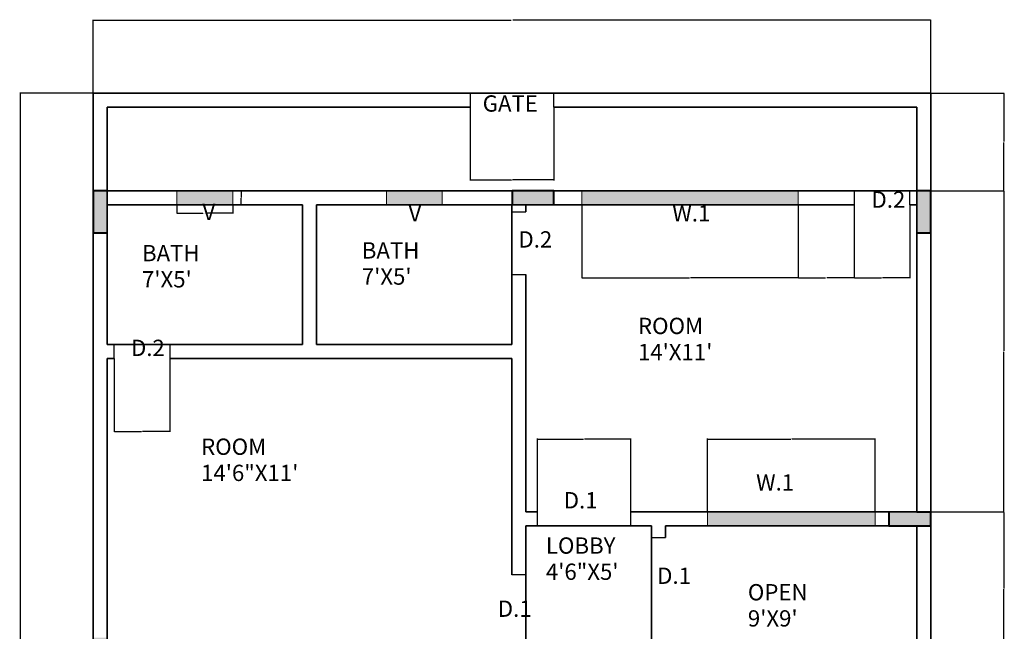
# Model space of a CAD drawing. Units: inches. Extents: x 2156 to 3149, y 1513 to 2286.
# Tile 2 of 5: x 2156 to 2579, y 1937 to 2200. Entities that reach past the tile are written whole.
import ezdxf

# ---------------------------------------------------------------- set-up
doc = ezdxf.new("R2010")
doc.units = ezdxf.units.IN
for name, color, linetype, lineweight in [('A-ANNO-DIMS', 2, 'Continuous', 18), ('A-ANNO-TEXT', 7, 'Continuous', 18), ('A-AREA-IDEN', 7, 'Continuous', 18), ('A-COLS', 7, 'Continuous', 40), ('A-COLS-PATT', 18, 'Continuous', 13), ('A-DOOR', 3, 'Continuous', 25), ('A-GLAZ', 4, 'Continuous', 18), ('A-GLAZ-PATT', 252, 'Continuous', 13), ('A-SITE-GATE', 3, 'Continuous', 25), ('A-SITE-WALL', 7, 'Continuous', 35), ('A-WALL', 7, 'Continuous', 35)]:
    doc.layers.add(name, color=color, linetype=linetype, lineweight=lineweight)
doc.styles.get("Standard").update_dxf_attribs({"font": 'arial.ttf'})
doc.dimstyles.get("Standard").update_dxf_attribs({"dimtxt": 0.18, "dimasz": 0.18, "dimexe": 0.18, "dimexo": 0.0625, "dimgap": 0.09, "dimtad": 0, "dimtih": 1, "dimtoh": 1, "dimdec": 4, "dimzin": 0, "dimdsep": 46, "dimtxsty": 'Standard', "dimcen": 0.09, "dimadec": 0, "dimazin": 0, "dimtfac": 1, "dimtdec": 4, "dimtofl": 0, "dimtmove": 0, "dimatfit": 3, "dimfxl": 1, "dimtolj": 1, "dimtzin": 0, "dimarcsym": 0})

# ---------------------------------------------------------------- blocks, each defined once
blk = doc.blocks.new('COL-6X18-PLAN')
for p, q in [((6, 18), (0, 18)), ((0, 18), (0, 0)), ((0, 0), (6, 0))]:
    blk.add_line(p, q)
blk = doc.blocks.new('VENT-24-PLAN')
for p, q in [((0, 0), (0, 6)), ((0, 6), (24, 6)), ((24, 6), (24, 0))]:
    blk.add_line(p, q)
blk = doc.blocks.new('*D9')
at = {"layer": 'A-ANNO-DIMS', "color": 0, "lineweight": -2, "transparency": 16777216}
for p, q in [((2223.92, 2120.47), (2223.92, 2116.76)), ((2247.92, 2120.47), (2247.92, 2116.76)), ((2224.1, 2116.94), (2235.02, 2116.94)), ((2247.74, 2116.94), (2236.82, 2116.94))]:
    blk.add_line(p, q, dxfattribs=at)
at = {"layer": 'A-ANNO-DIMS', "color": 0, "transparency": 16777216}
for points in [[(2224.1, 2116.97), (2224.1, 2116.91), (2223.92, 2116.94)], [(2247.74, 2116.97), (2247.74, 2116.91), (2247.92, 2116.94)]]:
    blk.add_solid(points, dxfattribs=at)
at = {"layer": 'Defpoints', "color": 0, "transparency": 16777216}
for p in [(2223.92, 2120.54), (2247.92, 2120.54), (2247.92, 2116.94)]:
    blk.add_point(p, dxfattribs=at)
at = {"layer": 'A-ANNO-DIMS', "color": 0, "transparency": 16777216, "insert": (2235.92, 2116.94), "char_height": 0.18, "attachment_point": 5}
blk.add_mtext('\\A1;VENT 24 TYP.', dxfattribs=at)
blk = doc.blocks.new('*D10')
at = {"layer": 'A-ANNO-DIMS', "color": 0, "lineweight": -2, "transparency": 16777216}
for p, q in [((2247.98, 2126.54), (2251.7, 2126.54)), ((2251.52, 2126.36), (2251.52, 2123.72)), ((2247.98, 2120.54), (2251.7, 2120.54)), ((2251.52, 2120.72), (2251.52, 2123.35))]:
    blk.add_line(p, q, dxfattribs=at)
at = {"layer": 'A-ANNO-DIMS', "color": 0, "transparency": 16777216}
for points in [[(2251.49, 2126.36), (2251.55, 2126.36), (2251.52, 2126.54)], [(2251.49, 2120.72), (2251.55, 2120.72), (2251.52, 2120.54)]]:
    blk.add_solid(points, dxfattribs=at)
at = {"layer": 'Defpoints', "color": 0, "transparency": 16777216}
for p in [(2247.92, 2126.54), (2251.52, 2126.54), (2247.92, 2120.54)]:
    blk.add_point(p, dxfattribs=at)
at = {"layer": 'A-ANNO-DIMS', "color": 0, "transparency": 16777216, "insert": (2251.52, 2123.54), "char_height": 0.18, "attachment_point": 5}
blk.add_mtext('\\A1;6 TYP.', dxfattribs=at)
blk = doc.blocks.new('*D19')
at = {"layer": 'A-ANNO-DIMS', "color": 0, "lineweight": -2, "transparency": 16777216}
for p, q in [((2187.92, 2168.6), (2187.92, 2200.07)), ((2188.1, 2199.89), (2367.63, 2199.89)), ((2547.74, 2199.89), (2368.21, 2199.89)), ((2547.92, 2168.6), (2547.92, 2200.07))]:
    blk.add_line(p, q, dxfattribs=at)
at = {"layer": 'A-ANNO-DIMS', "color": 0, "transparency": 16777216}
for points in [[(2188.1, 2199.92), (2188.1, 2199.86), (2187.92, 2199.89)], [(2547.74, 2199.92), (2547.74, 2199.86), (2547.92, 2199.89)]]:
    blk.add_solid(points, dxfattribs=at)
at = {"layer": 'Defpoints', "color": 0, "transparency": 16777216}
for p in [(2547.92, 2199.89), (2187.92, 2168.54), (2547.92, 2168.54)]:
    blk.add_point(p, dxfattribs=at)
at = {"layer": 'A-ANNO-DIMS', "color": 0, "transparency": 16777216, "insert": (2367.92, 2199.89), "char_height": 0.18, "attachment_point": 5}
blk.add_mtext('\\A1;360', dxfattribs=at)
blk = doc.blocks.new('*D24')
at = {"layer": 'A-ANNO-DIMS', "color": 0, "lineweight": -2, "transparency": 16777216}
for p, q in [((2187.86, 2168.54), (2156.39, 2168.54)), ((2156.57, 2168.36), (2156.57, 1856.72)), ((2156.57, 1544.72), (2156.57, 1856.35)), ((2187.86, 1544.54), (2156.39, 1544.54))]:
    blk.add_line(p, q, dxfattribs=at)
at = {"layer": 'A-ANNO-DIMS', "color": 0, "transparency": 16777216}
for points in [[(2156.54, 2168.36), (2156.6, 2168.36), (2156.57, 2168.54)], [(2156.54, 1544.72), (2156.6, 1544.72), (2156.57, 1544.54)]]:
    blk.add_solid(points, dxfattribs=at)
at = {"layer": 'Defpoints', "color": 0, "transparency": 16777216}
for p in [(2156.57, 2168.54), (2187.92, 2168.54), (2187.92, 1544.54)]:
    blk.add_point(p, dxfattribs=at)
at = {"layer": 'A-ANNO-DIMS', "color": 0, "transparency": 16777216, "insert": (2156.57, 1856.54), "char_height": 0.18, "attachment_point": 5}
blk.add_mtext('\\A1;624', dxfattribs=at)
blk = doc.blocks.new('*D29')
at = {"layer": 'A-ANNO-DIMS', "color": 0, "lineweight": -2, "transparency": 16777216}
for p, q in [((2547.98, 1988.54), (2579.45, 1988.54)), ((2579.27, 1988.36), (2579.27, 1955.72)), ((2579.27, 1922.72), (2579.27, 1955.35)), ((2433.98, 1922.54), (2579.45, 1922.54))]:
    blk.add_line(p, q, dxfattribs=at)
at = {"layer": 'A-ANNO-DIMS', "color": 0, "transparency": 16777216}
for points in [[(2579.24, 1988.36), (2579.3, 1988.36), (2579.27, 1988.54)], [(2579.24, 1922.72), (2579.3, 1922.72), (2579.27, 1922.54)]]:
    blk.add_solid(points, dxfattribs=at)
at = {"layer": 'Defpoints', "color": 0, "transparency": 16777216}
for p in [(2547.92, 1988.54), (2579.27, 1988.54), (2433.92, 1922.54)]:
    blk.add_point(p, dxfattribs=at)
at = {"layer": 'A-ANNO-DIMS', "color": 0, "transparency": 16777216, "insert": (2579.27, 1955.54), "char_height": 0.18, "attachment_point": 5}
blk.add_mtext('\\A1;66', dxfattribs=at)
blk = doc.blocks.new('*D30')
at = {"layer": 'A-ANNO-DIMS', "color": 0, "lineweight": -2, "transparency": 16777216}
for p, q in [((2547.98, 2126.54), (2579.45, 2126.54)), ((2579.27, 2126.36), (2579.27, 2057.72)), ((2579.27, 1988.72), (2579.27, 2057.35)), ((2547.98, 1988.54), (2579.45, 1988.54))]:
    blk.add_line(p, q, dxfattribs=at)
at = {"layer": 'A-ANNO-DIMS', "color": 0, "transparency": 16777216}
for points in [[(2579.24, 2126.36), (2579.3, 2126.36), (2579.27, 2126.54)], [(2579.24, 1988.72), (2579.3, 1988.72), (2579.27, 1988.54)]]:
    blk.add_solid(points, dxfattribs=at)
at = {"layer": 'Defpoints', "color": 0, "transparency": 16777216}
for p in [(2547.92, 2126.54), (2579.27, 2126.54), (2547.92, 1988.54)]:
    blk.add_point(p, dxfattribs=at)
at = {"layer": 'A-ANNO-DIMS', "color": 0, "transparency": 16777216, "insert": (2579.27, 2057.54), "char_height": 0.18, "attachment_point": 5}
blk.add_mtext('\\A1;138', dxfattribs=at)
blk = doc.blocks.new('*D31')
at = {"layer": 'A-ANNO-DIMS', "color": 0, "lineweight": -2, "transparency": 16777216}
for p, q in [((2547.98, 2168.54), (2579.45, 2168.54)), ((2579.27, 2168.36), (2579.27, 2147.72)), ((2579.27, 2126.72), (2579.27, 2147.36)), ((2547.98, 2126.54), (2579.45, 2126.54))]:
    blk.add_line(p, q, dxfattribs=at)
at = {"layer": 'A-ANNO-DIMS', "color": 0, "transparency": 16777216}
for points in [[(2579.24, 2168.36), (2579.3, 2168.36), (2579.27, 2168.54)], [(2579.24, 2126.72), (2579.3, 2126.72), (2579.27, 2126.54)]]:
    blk.add_solid(points, dxfattribs=at)
at = {"layer": 'Defpoints', "color": 0, "transparency": 16777216}
for p in [(2547.92, 2168.54), (2579.27, 2168.54), (2547.92, 2126.54)]:
    blk.add_point(p, dxfattribs=at)
at = {"layer": 'A-ANNO-DIMS', "color": 0, "transparency": 16777216, "insert": (2579.27, 2147.54), "char_height": 0.18, "attachment_point": 5}
blk.add_mtext('\\A1;42', dxfattribs=at)
blk = doc.blocks.new('*D32')
at = {"layer": 'A-ANNO-DIMS', "color": 0, "lineweight": -2, "transparency": 16777216}
for p, q in [((2349.92, 2162.47), (2349.92, 2131.01)), ((2385.92, 2162.47), (2385.92, 2131.01)), ((2350.1, 2131.19), (2367.7, 2131.19)), ((2385.74, 2131.19), (2368.14, 2131.19))]:
    blk.add_line(p, q, dxfattribs=at)
at = {"layer": 'A-ANNO-DIMS', "color": 0, "transparency": 16777216}
for points in [[(2350.1, 2131.22), (2350.1, 2131.16), (2349.92, 2131.19)], [(2385.74, 2131.22), (2385.74, 2131.16), (2385.92, 2131.19)]]:
    blk.add_solid(points, dxfattribs=at)
at = {"layer": 'Defpoints', "color": 0, "transparency": 16777216}
for p in [(2349.92, 2162.54), (2385.92, 2162.54), (2349.92, 2131.19)]:
    blk.add_point(p, dxfattribs=at)
at = {"layer": 'A-ANNO-DIMS', "color": 0, "transparency": 16777216, "insert": (2367.92, 2131.19), "char_height": 0.18, "attachment_point": 5}
blk.add_mtext('\\A1;36', dxfattribs=at)
blk = doc.blocks.new('*D33')
at = {"layer": 'A-ANNO-DIMS', "color": 0, "lineweight": -2, "transparency": 16777216}
for p, q in [((2397.92, 2120.47), (2397.92, 2089.01)), ((2490.92, 2120.47), (2490.92, 2089.01)), ((2398.1, 2089.19), (2444.2, 2089.19)), ((2490.74, 2089.19), (2444.64, 2089.19))]:
    blk.add_line(p, q, dxfattribs=at)
at = {"layer": 'A-ANNO-DIMS', "color": 0, "transparency": 16777216}
for points in [[(2398.1, 2089.22), (2398.1, 2089.16), (2397.92, 2089.19)], [(2490.74, 2089.22), (2490.74, 2089.16), (2490.92, 2089.19)]]:
    blk.add_solid(points, dxfattribs=at)
at = {"layer": 'Defpoints', "color": 0, "transparency": 16777216}
for p in [(2397.92, 2120.54), (2490.92, 2120.54), (2397.92, 2089.19)]:
    blk.add_point(p, dxfattribs=at)
at = {"layer": 'A-ANNO-DIMS', "color": 0, "transparency": 16777216, "insert": (2444.42, 2089.19), "char_height": 0.18, "attachment_point": 5}
blk.add_mtext('\\A1;93', dxfattribs=at)
blk = doc.blocks.new('*D34')
at = {"layer": 'A-ANNO-DIMS', "color": 0, "lineweight": -2, "transparency": 16777216}
for p, q in [((2490.92, 2120.47), (2490.92, 2089.01)), ((2514.92, 2120.47), (2514.92, 2089.01)), ((2491.1, 2089.19), (2502.7, 2089.19)), ((2514.74, 2089.19), (2503.14, 2089.19))]:
    blk.add_line(p, q, dxfattribs=at)
at = {"layer": 'A-ANNO-DIMS', "color": 0, "transparency": 16777216}
for points in [[(2491.1, 2089.22), (2491.1, 2089.16), (2490.92, 2089.19)], [(2514.74, 2089.22), (2514.74, 2089.16), (2514.92, 2089.19)]]:
    blk.add_solid(points, dxfattribs=at)
at = {"layer": 'Defpoints', "color": 0, "transparency": 16777216}
for p in [(2490.92, 2120.54), (2514.92, 2120.54), (2490.92, 2089.19)]:
    blk.add_point(p, dxfattribs=at)
at = {"layer": 'A-ANNO-DIMS', "color": 0, "transparency": 16777216, "insert": (2502.92, 2089.19), "char_height": 0.18, "attachment_point": 5}
blk.add_mtext('\\A1;24', dxfattribs=at)
blk = doc.blocks.new('*D35')
at = {"layer": 'A-ANNO-DIMS', "color": 0, "lineweight": -2, "transparency": 16777216}
for p, q in [((2514.92, 2120.47), (2514.92, 2089.01)), ((2538.92, 2120.47), (2538.92, 2089.01)), ((2515.1, 2089.19), (2526.7, 2089.19)), ((2538.74, 2089.19), (2527.14, 2089.19))]:
    blk.add_line(p, q, dxfattribs=at)
at = {"layer": 'A-ANNO-DIMS', "color": 0, "transparency": 16777216}
for points in [[(2515.1, 2089.22), (2515.1, 2089.16), (2514.92, 2089.19)], [(2538.74, 2089.22), (2538.74, 2089.16), (2538.92, 2089.19)]]:
    blk.add_solid(points, dxfattribs=at)
at = {"layer": 'Defpoints', "color": 0, "transparency": 16777216}
for p in [(2514.92, 2120.54), (2538.92, 2120.54), (2514.92, 2089.19)]:
    blk.add_point(p, dxfattribs=at)
at = {"layer": 'A-ANNO-DIMS', "color": 0, "transparency": 16777216, "insert": (2526.92, 2089.19), "char_height": 0.18, "attachment_point": 5}
blk.add_mtext('\\A1;24', dxfattribs=at)
blk = doc.blocks.new('*D36')
at = {"layer": 'A-ANNO-DIMS', "color": 0, "lineweight": -2, "transparency": 16777216}
for p, q in [((2451.92, 1988.6), (2451.92, 2020.07)), ((2452.1, 2019.89), (2487.7, 2019.89)), ((2523.74, 2019.89), (2488.14, 2019.89)), ((2523.92, 1988.6), (2523.92, 2020.07))]:
    blk.add_line(p, q, dxfattribs=at)
at = {"layer": 'A-ANNO-DIMS', "color": 0, "transparency": 16777216}
for points in [[(2452.1, 2019.92), (2452.1, 2019.86), (2451.92, 2019.89)], [(2523.74, 2019.92), (2523.74, 2019.86), (2523.92, 2019.89)]]:
    blk.add_solid(points, dxfattribs=at)
at = {"layer": 'Defpoints', "color": 0, "transparency": 16777216}
for p in [(2523.92, 2019.89), (2451.92, 1988.54), (2523.92, 1988.54)]:
    blk.add_point(p, dxfattribs=at)
at = {"layer": 'A-ANNO-DIMS', "color": 0, "transparency": 16777216, "insert": (2487.92, 2019.89), "char_height": 0.18, "attachment_point": 5}
blk.add_mtext('\\A1;72', dxfattribs=at)
blk = doc.blocks.new('*D37')
at = {"layer": 'A-ANNO-DIMS', "color": 0, "lineweight": -2, "transparency": 16777216}
for p, q in [((2378.92, 1988.6), (2378.92, 2020.07)), ((2379.1, 2019.89), (2398.7, 2019.89)), ((2418.74, 2019.89), (2399.14, 2019.89)), ((2418.92, 1988.6), (2418.92, 2020.07))]:
    blk.add_line(p, q, dxfattribs=at)
at = {"layer": 'A-ANNO-DIMS', "color": 0, "transparency": 16777216}
for points in [[(2379.1, 2019.92), (2379.1, 2019.86), (2378.92, 2019.89)], [(2418.74, 2019.92), (2418.74, 2019.86), (2418.92, 2019.89)]]:
    blk.add_solid(points, dxfattribs=at)
at = {"layer": 'Defpoints', "color": 0, "transparency": 16777216}
for p in [(2418.92, 2019.89), (2378.92, 1988.54), (2418.92, 1988.54)]:
    blk.add_point(p, dxfattribs=at)
at = {"layer": 'A-ANNO-DIMS', "color": 0, "transparency": 16777216, "insert": (2398.92, 2019.89), "char_height": 0.18, "attachment_point": 5}
blk.add_mtext('\\A1;40', dxfattribs=at)
blk = doc.blocks.new('*D38')
at = {"layer": 'A-ANNO-DIMS', "color": 0, "lineweight": -2, "transparency": 16777216}
for p, q in [((2196.92, 2054.47), (2196.92, 2023.01)), ((2220.92, 2054.47), (2220.92, 2023.01)), ((2197.1, 2023.19), (2208.7, 2023.19)), ((2220.74, 2023.19), (2209.14, 2023.19))]:
    blk.add_line(p, q, dxfattribs=at)
at = {"layer": 'A-ANNO-DIMS', "color": 0, "transparency": 16777216}
for points in [[(2197.1, 2023.22), (2197.1, 2023.16), (2196.92, 2023.19)], [(2220.74, 2023.22), (2220.74, 2023.16), (2220.92, 2023.19)]]:
    blk.add_solid(points, dxfattribs=at)
at = {"layer": 'Defpoints', "color": 0, "transparency": 16777216}
for p in [(2196.92, 2054.54), (2220.92, 2054.54), (2196.92, 2023.19)]:
    blk.add_point(p, dxfattribs=at)
at = {"layer": 'A-ANNO-DIMS', "color": 0, "transparency": 16777216, "insert": (2208.92, 2023.19), "char_height": 0.18, "attachment_point": 5}
blk.add_mtext('\\A1;24', dxfattribs=at)

msp = doc.modelspace()

# ---------------------------------------------------------------- hatches: boundary and pattern name
at = {"layer": 'A-COLS-PATT'}
h = msp.add_hatch(color=256, dxfattribs=at)
h.dxf.hatch_style = 1
h.paths.add_polyline_path([(2193.921, 2120.536), (2193.921, 2126.536), (2187.921, 2126.536), (2187.921, 2108.536), (2193.921, 2108.536)])
h.paths.add_polyline_path([(2385.921, 2126.536), (2367.921, 2126.536), (2367.921, 2120.536), (2373.921, 2120.536), (2385.921, 2120.536)])
h.paths.add_polyline_path([(2547.921, 2126.536), (2541.921, 2126.536), (2541.921, 2108.536), (2547.921, 2108.536)])
h.paths.add_polyline_path([(2547.921, 1988.536), (2541.921, 1988.536), (2541.921, 1982.536), (2547.921, 1982.536)])
h.paths.add_polyline_path([(2541.921, 1988.536), (2529.921, 1988.536), (2529.921, 1982.536), (2541.921, 1982.536)])
h.paths.add_polyline_path([(2373.921, 1922.536), (2367.921, 1922.536), (2355.921, 1922.536), (2355.921, 1916.536), (2373.921, 1916.536)])
h.paths.add_polyline_path([(2193.921, 1934.536), (2187.921, 1934.536), (2187.921, 1916.536), (2193.921, 1916.536)])
h.paths.add_polyline_path([(2433.921, 1880.536), (2427.921, 1880.536), (2427.921, 1871.536), (2427.921, 1862.536), (2433.921, 1862.536)])
h.paths.add_polyline_path([(2241.921, 1772.536), (2235.921, 1772.536), (2235.921, 1760.536), (2235.921, 1754.536), (2241.921, 1754.536)])
h.paths.add_polyline_path([(2443.921, 1760.536), (2433.921, 1760.536), (2427.921, 1760.536), (2425.921, 1760.536), (2425.921, 1754.536), (2443.921, 1754.536)])
h.paths.add_polyline_path([(2547.921, 1760.536), (2541.921, 1760.536), (2541.921, 1754.536), (2541.921, 1742.536), (2547.921, 1742.536)])
at = {"layer": 'A-GLAZ-PATT'}
h = msp.add_hatch(color=256, dxfattribs=at)
h.dxf.hatch_style = 1
h.paths.add_polyline_path([(2490.921, 2126.536), (2397.921, 2126.536), (2397.921, 2120.536), (2490.921, 2120.536)])
h.paths.add_polyline_path([(2337.921, 2126.536), (2313.921, 2126.536), (2313.921, 2120.536), (2325.921, 2120.536), (2337.921, 2120.536)])
h.paths.add_polyline_path([(2247.921, 2126.536), (2223.921, 2126.536), (2223.921, 2120.536), (2235.921, 2120.536), (2247.921, 2120.536)])
h.paths.add_polyline_path([(2241.921, 1891.536), (2235.921, 1891.536), (2235.921, 1831.536), (2241.921, 1831.536), (2241.921, 1861.536)])
h.paths.add_polyline_path([(2235.921, 1922.536), (2193.921, 1922.536), (2193.921, 1916.536), (2235.921, 1916.536)])
h.paths.add_polyline_path([(2505.921, 1874.536), (2469.921, 1874.536), (2469.921, 1868.536), (2505.921, 1868.536)])
h.paths.add_polyline_path([(2523.921, 1988.536), (2451.921, 1988.536), (2451.921, 1982.536), (2523.921, 1982.536)])
h.paths.add_polyline_path([(2307.921, 1760.536), (2289.921, 1760.536), (2289.921, 1754.536), (2298.921, 1754.536), (2307.921, 1754.536)])
h.paths.add_polyline_path([(2422.921, 1760.536), (2404.921, 1760.536), (2404.921, 1754.536), (2413.921, 1754.536), (2422.921, 1754.536)])

# ---------------------------------------------------------------- linework, layer by layer
at = {"layer": 'A-COLS'}
msp.add_line((2541.921, 1988.536), (2547.921, 1988.536), dxfattribs=at)
at = {"layer": 'A-DOOR'}
for p, q in [((2538.921, 2126.536), (2514.921, 2126.536)), ((2514.921, 2126.536), (2514.921, 2120.536)), ((2538.921, 2120.536), (2538.921, 2126.536)), ((2367.921, 2117.536), (2373.921, 2117.536)), ((2367.921, 2117.536), (2367.921, 2090.536)), ((2367.921, 2090.536), (2373.921, 2090.536)), ((2196.921, 2054.536), (2196.921, 2060.536)), ((2196.921, 2060.536), (2214.921, 2060.536)), ((2214.921, 2060.536), (2220.921, 2060.536)), ((2220.921, 2060.536), (2220.921, 2054.536)), ((2378.921, 1982.536), (2378.921, 1988.536)), ((2418.921, 1982.536), (2418.921, 1988.536)), ((2427.921, 1977.536), (2433.921, 1977.536)), ((2373.921, 1961.536), (2367.921, 1961.536)), ((2373.921, 1925.536), (2373.921, 1961.536))]:
    msp.add_line(p, q, dxfattribs=at)
at = {"layer": 'A-GLAZ'}
for p, q in [((2397.921, 2120.536), (2397.921, 2126.536)), ((2490.921, 2120.536), (2490.921, 2126.536)), ((2451.921, 1982.536), (2451.921, 1988.536)), ((2523.921, 1982.536), (2523.921, 1988.536))]:
    msp.add_line(p, q, dxfattribs=at)
at = {"layer": 'A-SITE-GATE'}
for p, q in [((2385.921, 2168.536), (2349.921, 2168.536)), ((2349.921, 2168.536), (2349.921, 2162.536)), ((2385.921, 2162.536), (2385.921, 2168.536))]:
    msp.add_line(p, q, dxfattribs=at)
at = {"layer": 'A-SITE-WALL'}
for p, q in [((2187.921, 2168.536), (2547.921, 2168.536)), ((2187.921, 1544.536), (2187.921, 2168.536)), ((2187.921, 2168.536), (2193.921, 2168.536)), ((2547.921, 2168.536), (2547.921, 1544.536)), ((2193.921, 2162.536), (2349.921, 2162.536)), ((2193.921, 2162.536), (2193.921, 2126.536)), ((2193.921, 2060.536), (2193.921, 2162.536)), ((2367.921, 2162.536), (2367.921, 2162.536)), ((2385.921, 2162.536), (2541.921, 2162.536)), ((2541.921, 2162.536), (2541.921, 1988.536))]:
    msp.add_line(p, q, dxfattribs=at)
at = {"layer": 'A-WALL'}
for p, q in [((2193.921, 2126.536), (2541.921, 2126.536)), ((2541.921, 2126.536), (2541.921, 2120.536)), ((2193.921, 2060.536), (2193.921, 2120.536)), ((2193.921, 2120.536), (2277.921, 2120.536)), ((2193.921, 2120.536), (2277.921, 2120.536)), ((2235.921, 2120.536), (2223.921, 2120.536)), ((2277.921, 2120.536), (2235.921, 2120.536)), ((2277.921, 2120.536), (2277.921, 2060.536)), ((2283.921, 2060.536), (2283.921, 2120.536)), ((2283.921, 2120.536), (2367.921, 2120.536)), ((2367.921, 2120.536), (2283.921, 2120.536)), ((2367.921, 2120.536), (2283.921, 2120.536)), ((2283.921, 2120.536), (2325.921, 2120.536)), ((2325.921, 2120.536), (2313.921, 2120.536)), ((2373.921, 2120.536), (2367.921, 2120.536)), ((2367.921, 2120.536), (2367.921, 2060.536)), ((2367.921, 2120.536), (2367.921, 2117.536)), ((2367.921, 2099.536), (2367.921, 2120.536)), ((2373.921, 2120.536), (2373.921, 2117.536)), ((2373.921, 2120.536), (2385.921, 2120.536)), ((2514.921, 2120.536), (2373.921, 2120.536)), ((2514.921, 2120.536), (2373.921, 2120.536)), ((2385.921, 2120.536), (2397.921, 2120.536)), ((2514.921, 2120.536), (2490.921, 2120.536)), ((2541.921, 2120.536), (2538.921, 2120.536)), ((2541.921, 2120.536), (2538.921, 2120.536)), ((2541.921, 2120.536), (2538.921, 2120.536)), ((2541.921, 1988.536), (2541.921, 2120.536)), ((2373.921, 2090.536), (2373.921, 1988.536)), ((2277.921, 2060.536), (2193.921, 2060.536)), ((2367.921, 2060.536), (2283.921, 2060.536)), ((2193.921, 2054.536), (2196.921, 2054.536)), ((2193.921, 1760.536), (2193.921, 2054.536)), ((2193.921, 2054.536), (2193.921, 2054.536)), ((2193.921, 2054.536), (2193.921, 2054.536)), ((2193.921, 2054.536), (2196.921, 2054.536)), ((2220.921, 2054.536), (2367.921, 2054.536)), ((2367.921, 2054.536), (2367.921, 1961.536)), ((2373.921, 1988.536), (2378.921, 1988.536)), ((2418.921, 1988.536), (2541.921, 1988.536)), ((2427.921, 1982.536), (2373.921, 1982.536)), ((2373.921, 1982.536), (2373.921, 1922.536)), ((2373.921, 1982.536), (2378.921, 1982.536)), ((2427.921, 1982.536), (2418.921, 1982.536)), ((2427.921, 1922.536), (2427.921, 1982.536)), ((2427.921, 1982.536), (2427.921, 1977.536)), ((2541.921, 1982.536), (2433.921, 1982.536)), ((2433.921, 1982.536), (2433.921, 1977.536)), ((2433.921, 1982.536), (2445.921, 1982.536)), ((2433.921, 1982.536), (2445.921, 1982.536)), ((2445.921, 1982.536), (2451.921, 1982.536)), ((2529.921, 1982.536), (2523.921, 1982.536)), ((2541.921, 1982.536), (2541.921, 1874.536))]:
    msp.add_line(p, q, dxfattribs=at)

# ---------------------------------------------------------------- block references
at = {"layer": 'A-COLS'}
msp.add_blockref('COL-6X18-PLAN', (2187.921, 2108.536), dxfattribs=at)
for p, rotation in [((2367.922, 2126.536), 270), ((2547.921, 2126.535), 180), ((2547.921, 1982.535), 89.99999999999999)]:
    msp.add_blockref('COL-6X18-PLAN', p, dxfattribs=dict(at, rotation=rotation))
at = {"layer": 'A-GLAZ'}
for p in [(2223.921, 2120.536), (2313.921, 2120.536)]:
    msp.add_blockref('VENT-24-PLAN', p, dxfattribs=at)

# ---------------------------------------------------------------- texts
at = {"layer": 'A-ANNO-TEXT'}
for s, p in [('GATE', (2355.334, 2160.555)), ('D.2', (2522.404, 2119.264)), ('V', (2234.902, 2113.955)), ('V', (2323.455, 2113.365)), ('W.1', (2436.803, 2113.365)), ('D.2', (2370.683, 2102.157)), ('D.2', (2204.204, 2055.557)), ('W.1', (2472.814, 1997.749)), ('D.1', (2390.165, 1990.081)), ('D.1', (2430.309, 1957.638)), ('D.1', (2361.828, 1943.481))]:
    msp.add_text(s, height=7, dxfattribs=at).set_placement(p)
at = {"layer": 'A-AREA-IDEN'}
for s, p in [('BATH', (2208.926, 2096.258)), ('BATH', (2303.383, 2097.438)), ("7'X5'", (2208.926, 2085.014)), ("7'X5'", (2303.383, 2086.193)), ('ROOM', (2422.044, 2064.995)), ("14'X11'", (2422.044, 2053.75)), ('ROOM', (2234.312, 2013.086)), ('14\'6"X11\'', (2234.312, 2001.841)), ('LOBBY', (2382.49, 1970.615)), ('4\'6"X5\'', (2382.49, 1959.37)), ('OPEN', (2469.272, 1950.559)), ("9'X9'", (2469.272, 1939.314))]:
    msp.add_text(s, height=7, dxfattribs=at).set_placement(p)

# ---------------------------------------------------------------- dimensions: what is measured, and where the dimension line sits
at = {"layer": 'A-ANNO-DIMS'}
for base, p1, p2, picture, middle in [((2547.921, 2199.886), (2187.921, 2168.536), (2547.921, 2168.536), '*D19', (2367.921, 2199.886)), ((2418.921, 2019.886), (2378.921, 1988.536), (2418.921, 1988.536), '*D37', (2398.921, 2019.886)), ((2523.921, 2019.886), (2451.921, 1988.536), (2523.921, 1988.536), '*D36', (2487.921, 2019.886))]:
    dim = msp.add_linear_dim(base=base, p1=p1, p2=p2, dimstyle='Standard', override={"dimdec": 0, "dimlfac": 1, "dimrnd": 0, "dimzin": 0, "dimdsep": 46, "dimlunit": 2}, dxfattribs=at)
    dim.commit()
    dim.dimension.update_dxf_attribs({"geometry": picture, "text_midpoint": middle})
for base, p1, p2, angle, picture, middle in [((2156.571, 2168.536), (2187.921, 1544.536), (2187.921, 2168.536), 90, '*D24', (2156.571, 1856.536)), ((2579.271, 2168.536), (2547.921, 2126.536), (2547.921, 2168.536), 90, '*D31', (2579.271, 2147.536)), ((2349.921, 2131.186), (2385.921, 2162.536), (2349.921, 2162.536), 180, '*D32', (2367.921, 2131.186)), ((2579.271, 2126.536), (2547.921, 1988.536), (2547.921, 2126.536), 90, '*D30', (2579.271, 2057.536)), ((2397.921, 2089.186), (2490.921, 2120.536), (2397.921, 2120.536), 180, '*D33', (2444.421, 2089.186)), ((2490.921, 2089.186), (2514.921, 2120.536), (2490.921, 2120.536), 180, '*D34', (2502.921, 2089.186)), ((2514.921, 2089.186), (2538.921, 2120.536), (2514.921, 2120.536), 180, '*D35', (2526.921, 2089.186)), ((2196.921, 2023.186), (2220.921, 2054.536), (2196.921, 2054.536), 180, '*D38', (2208.921, 2023.186)), ((2579.271, 1988.536), (2433.921, 1922.536), (2547.921, 1988.536), 90, '*D29', (2579.271, 1955.536))]:
    dim = msp.add_linear_dim(base=base, p1=p1, p2=p2, angle=angle, dimstyle='Standard', override={"dimdec": 0, "dimlfac": 1, "dimrnd": 0, "dimzin": 0, "dimdsep": 46, "dimlunit": 2}, dxfattribs=at)
    dim.commit()
    dim.dimension.update_dxf_attribs({"geometry": picture, "text_midpoint": middle})
dim = msp.add_linear_dim(base=(2251.521, 2126.536), p1=(2247.921, 2120.536), p2=(2247.921, 2126.536), angle=90, text='<> TYP.', dimstyle='Standard', override={"dimdec": 0, "dimlfac": 1, "dimrnd": 0, "dimzin": 0, "dimdsep": 46, "dimlunit": 2}, dxfattribs=at)
dim.commit()
dim.dimension.update_dxf_attribs({"geometry": '*D10', "text_midpoint": (2251.521, 2123.536)})
dim = msp.add_linear_dim(base=(2247.921, 2116.936), p1=(2223.921, 2120.536), p2=(2247.921, 2120.536), text='VENT <> TYP.', dimstyle='Standard', override={"dimdec": 0, "dimlfac": 1, "dimrnd": 0, "dimzin": 0, "dimdsep": 46, "dimlunit": 2}, dxfattribs=at)
dim.commit()
dim.dimension.update_dxf_attribs({"geometry": '*D9', "text_midpoint": (2235.921, 2116.936)})

doc.saveas('drawing.dxf')
